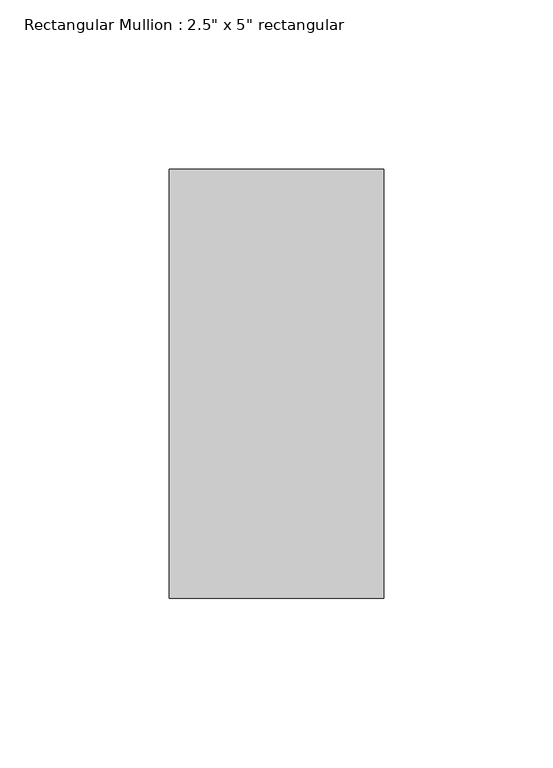
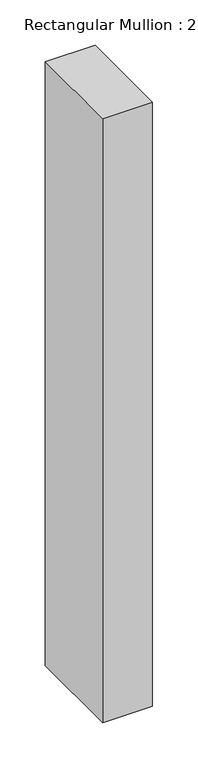
"""IFC4 building model written with IfcOpenShell, lengths in millimetres: member geometry."""

from ifc_helpers import new_model, si_unit, frame, origin, place, context, project, spatial, polyline, outline, extrude, source, transform, mapped, element, save


def member_5b006e0e(model_context):
    return source(origin(), model_context, "Body", "SweptSolid", [
        extrude(outline(polyline([(0.0, 63.5), (0.0, -63.5), (-63.5, -63.5), (-63.5, 63.5), (0.0, 63.5)])), frame((0.0, 0.0, -814.5761324), z_axis=(0.0, 0.0, 1.0), x_axis=(1.0, 0.0, 0.0)), (0.0, 0.0, 1.0), 814.5761324),
    ])


if __name__ == "__main__":
    model = new_model("IFC4")
    model_context = context("Model", 3, world=origin())
    ifc_project = project(units=[si_unit("LENGTHUNIT", "METRE", prefix="MILLI")], contexts=[model_context])
    site = spatial("IfcSite", under=ifc_project)
    building = spatial("IfcBuilding", under=site)
    placement = place(None, origin())
    member_shape = member_5b006e0e(model_context)
    element("IfcMember", 1, ObjectType="Rectangular Mullion : 2.5\" x 5\" rectangular", at=placement, inside=building, context=model_context, shape_type="MappedRepresentation", body=[
        mapped(member_shape, transform((0.0, 0.0, 0.0), x_axis=(1.0, 0.0, 0.0), y_axis=(0.0, 1.0, 0.0), z_axis=(0.0, 0.0, 1.0))),
    ])
    save(model, "model.ifc")

# Revit data of these elements
# Type "Rectangular Mullion : 2.5\" x 5\" rectangular"
#   built-in parameter 1007304 = 0.416667 (stored number, unit not read)
#   built-in parameter 1007301 = 0.104167 (stored number, unit not read)
#   built-in parameter 1007300 = 0.104167 (stored number, unit not read)
# Element 1 (IfcMember, "Rectangular Mullion : 2.5\" x 5\" rectangular")
#   Materials on its faces: "Aluminum"
# Materials
#   "Aluminum": class "Metal", colour RGB 247 247 247, transparency 0, Description = "Aluminum 6061", Cost = 0
